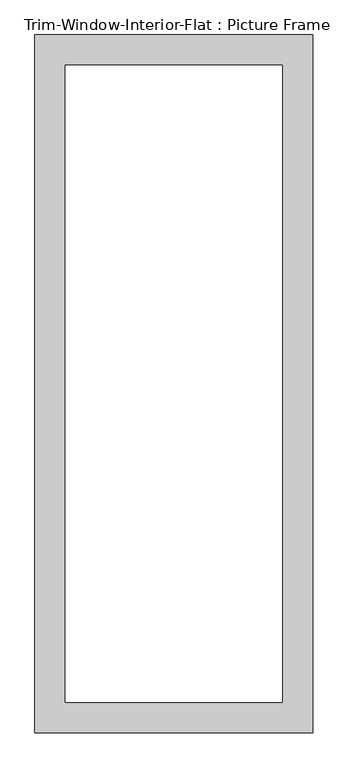
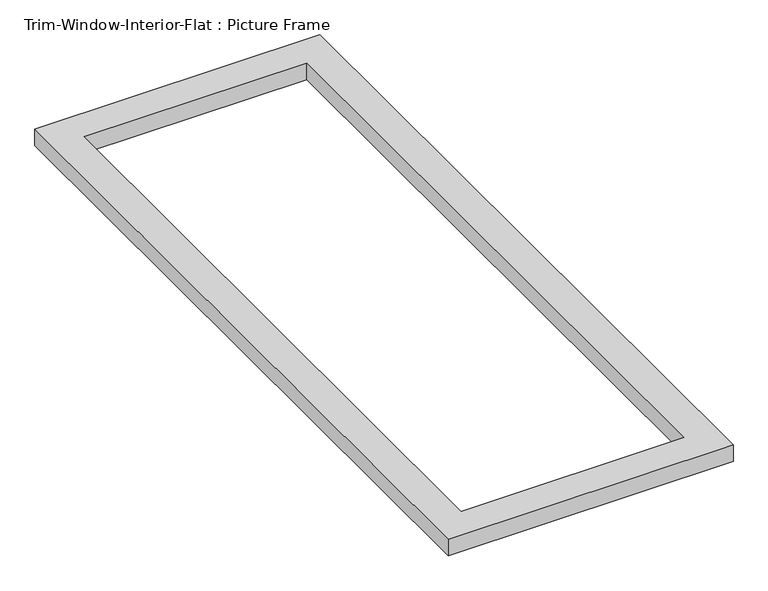
"""IFC4 building model written with IfcOpenShell, lengths in millimetres: proxy geometry, Trim-Window-Interior-Flat : Picture Frame."""

from ifc_helpers import new_model, si_unit, origin, origin_with_axes, place, context, project, spatial, polyline, outline, extrude, source, transform, mapped, element, save


def trim_window_interior_flat_picture_frame_a70901f7(model_context):
    return source(origin(), model_context, "Body", "SweptSolid", [
        extrude(outline(polyline([(260.35, 44.45), (260.35, -1263.65), (-260.35, -1263.65), (-260.35, 44.45), (260.35, 44.45)]), holes=[polyline([(203.2, -12.7), (-203.2, -12.7), (-203.2, -1206.5), (203.2, -1206.5), (203.2, -12.7)])]), origin_with_axes(), (0.0, 0.0, 1.0), 31.75),
    ])


if __name__ == "__main__":
    model = new_model("IFC4")
    model_context = context("Model", 3, world=origin())
    ifc_project = project(units=[si_unit("LENGTHUNIT", "METRE", prefix="MILLI")], contexts=[model_context])
    site = spatial("IfcSite", under=ifc_project)
    building = spatial("IfcBuilding", under=site)
    placement = place(None, origin())
    trim_window_interior_flat_picture_frame_shape = trim_window_interior_flat_picture_frame_a70901f7(model_context)
    element("IfcBuildingElementProxy", 1, Name="Trim-Window-Interior-Flat : Picture Frame", ObjectType="Trim-Window-Interior-Flat : Picture Frame", at=placement, inside=building, context=model_context, shape_type="MappedRepresentation", body=[
        mapped(trim_window_interior_flat_picture_frame_shape, transform((0.0, 0.0, 0.0), x_axis=(1.0, 0.0, 0.0), y_axis=(0.0, 1.0, 0.0), z_axis=(0.0, 0.0, 1.0))),
    ])
    save(model, "model.ifc")

# Revit data of these elements
# Type "Trim-Window-Interior-Flat : Picture Frame"
#   Trim Thickness_Picture Frame = 0' - 1 1/4"
#   Trim Width = 0' - 2 1/4"
#   Trim Thickness_with Sill = 0' - 0 3/4"
#   Sill Thickness = 0' - 1 1/4"
#   Opening Width [instance default] = 2' - 0"
#   Opening Height [instance default] = 3' - 0"
#   Default Elevation = 4' - 0"
#   Sill = no
#   Picture Frame = yes
#   Trim Material [instance default] = none
# Element 1 (IfcBuildingElementProxy, "Trim-Window-Interior-Flat : Picture Frame")
#   Opening Width = 1' - 5"
#   Opening Height = 4' - 0"
#   Trim Material = Wood - Stained
#   Materials on its faces: "Wood - Stained"
# Materials
#   "Wood - Stained": class "Wood", colour RGB 224 178 126, transparency 0, Cost = 0
